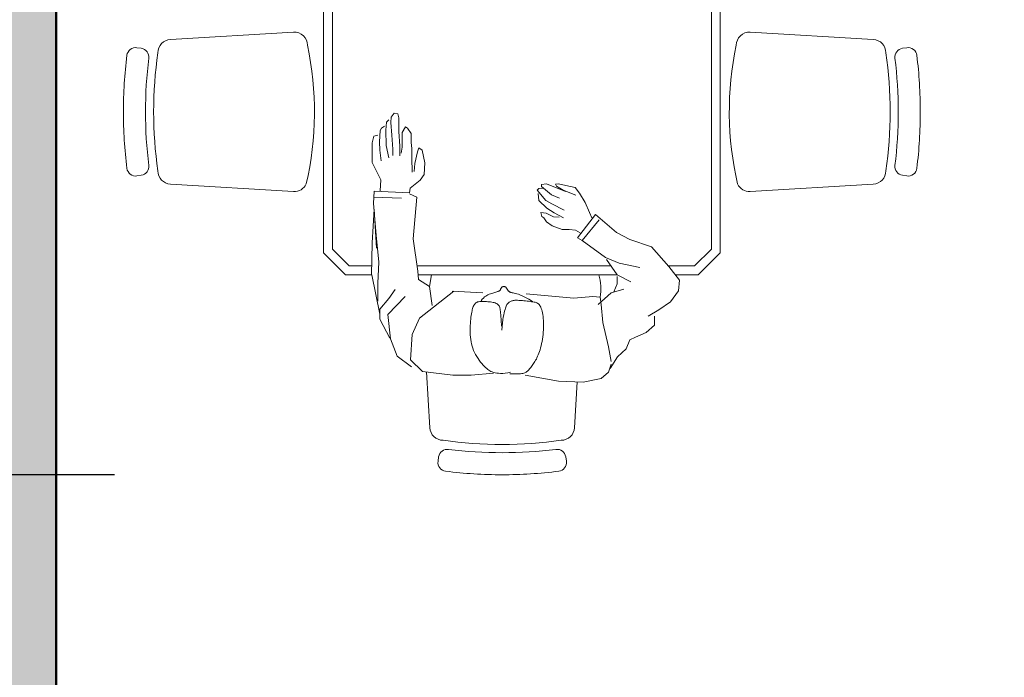
# Model space of a CAD drawing. Units: inches. Extents: x 1734 to 4011, y 1071 to 1891.
# Tile 19 of 27: x 3311 to 3379, y 1638 to 1683. Entities that reach past the tile are written whole.
import ezdxf

# ---------------------------------------------------------------- set-up
doc = ezdxf.new("R2010")
doc.units = ezdxf.units.IN
for name, color, linetype, lineweight in [('A-ANNO-DIMS', 2, 'Continuous', 18), ('A-FURN', 8, 'Continuous', 18), ('A-WALL', 7, 'Continuous', 50), ('A-WALL-PATT', 8, 'Continuous', 13)]:
    doc.layers.add(name, color=color, linetype=linetype, lineweight=lineweight)
doc.styles.get("Standard").update_dxf_attribs({"font": 'arial.ttf'})
doc.dimstyles.new('ISO-25', dxfattribs={"dimtxt": 5, "dimasz": 2.5, "dimexe": 1.25, "dimexo": 0.625, "dimtad": 1, "dimdec": 1, "dimlunit": 3, "dimtxsty": 'Standard', "dimcen": 2.5, "dimclrt": 1, "dimadec": 0, "dimazin": 0, "dimtfac": 1, "dimtdec": 1, "dimtmove": 0, "dimatfit": 3, "dimfxl": 1, "dimarcsym": 0})

# ---------------------------------------------------------------- blocks, each defined once
blk = doc.blocks.new('A$C421907B3')
for p, q in [((0.7079, 2.565), (0.7245, 2.5796)), ((0.7245, 2.5796), (0.7652, 2.5876)), ((0.7652, 2.5876), (0.8209, 2.5856)), ((0.8209, 2.5856), (0.8965, 2.5714)), ((0.9684, 2.5672), (1.0195, 2.5715)), ((1.0195, 2.5715), (1.0607, 2.5715)), ((1.0607, 2.5715), (1.1301, 2.5633)), ((0.7038, 2.5568), (0.6875, 2.5302)), ((0.7017, 2.5468), (0.7079, 2.565)), ((0.8792, 2.5478), (0.8777, 2.5455)), ((0.8808, 2.55), (0.8792, 2.5478)), ((0.8823, 2.5521), (0.8808, 2.55)), ((0.8839, 2.5541), (0.8823, 2.5521)), ((0.8853, 2.556), (0.8839, 2.5541)), ((0.8868, 2.5577), (0.8853, 2.556)), ((0.8883, 2.5594), (0.8868, 2.5577)), ((0.8897, 2.5609), (0.8883, 2.5594)), ((0.8911, 2.5623), (0.8897, 2.5609)), ((0.8926, 2.5635), (0.8911, 2.5623)), ((0.8941, 2.5647), (0.8926, 2.5635)), ((0.8958, 2.5657), (0.8941, 2.5647)), ((0.8976, 2.5665), (0.8958, 2.5657)), ((0.8996, 2.5672), (0.8976, 2.5665)), ((0.9018, 2.5678), (0.8996, 2.5672)), ((0.9043, 2.5682), (0.9018, 2.5678)), ((0.9071, 2.5684), (0.9043, 2.5682)), ((0.9102, 2.5686), (0.9071, 2.5684)), ((0.9137, 2.5687), (0.9102, 2.5686)), ((0.9175, 2.5687), (0.9137, 2.5687)), ((0.9217, 2.5687), (0.9175, 2.5687)), ((0.9264, 2.5687), (0.9217, 2.5687)), ((0.9314, 2.5687), (0.9264, 2.5687)), ((0.9361, 2.5662), (0.9297, 2.5647)), ((0.942, 2.5671), (0.9361, 2.5662)), ((0.9475, 2.5676), (0.942, 2.5671)), ((0.9525, 2.5677), (0.9475, 2.5676)), ((0.9571, 2.5675), (0.9525, 2.5677)), ((0.9614, 2.5669), (0.9571, 2.5675)), ((0.9652, 2.5662), (0.9614, 2.5669)), ((0.9686, 2.5653), (0.9652, 2.5662)), ((0.9717, 2.5643), (0.9686, 2.5653)), ((0.9745, 2.5632), (0.9717, 2.5643)), ((0.977, 2.5619), (0.9745, 2.5632)), ((0.9794, 2.5605), (0.977, 2.5619)), ((0.9818, 2.5588), (0.9794, 2.5605)), ((0.9841, 2.5568), (0.9818, 2.5588)), ((0.9865, 2.5545), (0.9841, 2.5568)), ((0.9891, 2.5519), (0.9865, 2.5545)), ((0.9918, 2.5489), (0.9891, 2.5519)), ((0.9948, 2.5455), (0.9918, 2.5489)), ((1.1301, 2.5633), (1.1567, 2.5368)), ((1.1546, 2.5531), (1.1875, 2.5285)), ((0.6875, 2.5302), (0.6672, 2.5117)), ((0.7017, 2.5405), (0.7079, 2.5077)), ((0.8669, 2.5256), (0.8655, 2.522)), ((0.8684, 2.5289), (0.8669, 2.5256)), ((0.8699, 2.5321), (0.8684, 2.5289)), ((0.8714, 2.5351), (0.8699, 2.5321)), ((0.873, 2.5379), (0.8714, 2.5351)), ((0.8745, 2.5405), (0.873, 2.5379)), ((0.8761, 2.543), (0.8745, 2.5405)), ((0.8777, 2.5455), (0.8761, 2.543)), ((0.9978, 2.5419), (0.9948, 2.5455)), ((1.0008, 2.5379), (0.9978, 2.5419)), ((1.0037, 2.5338), (1.0008, 2.5379)), ((1.0066, 2.5294), (1.0037, 2.5338)), ((1.0093, 2.5249), (1.0066, 2.5294)), ((1.1567, 2.5368), (1.153, 2.4792)), ((1.1875, 2.5285), (1.202, 2.4895)), ((0.6672, 2.5117), (0.6589, 2.4912)), ((0.7079, 2.5077), (0.7204, 2.4524)), ((0.8604, 2.5049), (0.8594, 2.5001)), ((0.8616, 2.5096), (0.8604, 2.5049)), ((0.8628, 2.514), (0.8616, 2.5096)), ((0.8641, 2.5181), (0.8628, 2.514)), ((0.8655, 2.522), (0.8641, 2.5181)), ((1.0117, 2.5203), (1.0093, 2.5249)), ((1.0138, 2.5155), (1.0117, 2.5203)), ((1.0156, 2.5107), (1.0138, 2.5155)), ((1.0171, 2.5058), (1.0156, 2.5107)), ((1.0184, 2.5008), (1.0171, 2.5058)), ((0.6464, 2.4852), (0.6219, 2.4749)), ((0.6589, 2.4912), (0.6464, 2.4852)), ((0.8568, 2.4847), (0.8562, 2.4794)), ((0.8576, 2.49), (0.8568, 2.4847)), ((0.8584, 2.4951), (0.8576, 2.49)), ((0.8594, 2.5001), (0.8584, 2.4951)), ((1.0194, 2.4958), (1.0184, 2.5008)), ((1.0202, 2.4907), (1.0194, 2.4958)), ((1.0208, 2.4855), (1.0202, 2.4907)), ((1.0212, 2.4802), (1.0208, 2.4855)), ((1.202, 2.4895), (1.2083, 2.4342)), ((1.2041, 2.4875), (1.2266, 2.4445)), ((0.6219, 2.4749), (0.6036, 2.4584)), ((0.6036, 2.4584), (0.6036, 2.4379)), ((0.8552, 2.4632), (0.8551, 2.4579)), ((0.8554, 2.4686), (0.8552, 2.4632)), ((0.8558, 2.474), (0.8554, 2.4686)), ((0.8562, 2.4794), (0.8558, 2.474)), ((0.9483, 2.453), (0.9491, 2.4609)), ((0.9491, 2.4609), (0.9498, 2.4698)), ((0.9505, 2.4603), (0.9511, 2.447)), ((1.021, 2.4541), (1.0212, 2.4591)), ((1.0214, 2.4749), (1.0212, 2.4802)), ((1.0212, 2.4591), (1.0214, 2.4643)), ((1.0215, 2.4696), (1.0214, 2.4749)), ((1.0214, 2.4643), (1.0215, 2.4696)), ((1.153, 2.4792), (1.1364, 2.4424)), ((0.6178, 2.4379), (0.5933, 2.4236)), ((0.7204, 2.4524), (0.7246, 2.4114)), ((0.8551, 2.4579), (0.8552, 2.4527)), ((0.8552, 2.4527), (0.8554, 2.4476)), ((0.8554, 2.4476), (0.8557, 2.4428)), ((0.8557, 2.4428), (0.8561, 2.4383)), ((0.8561, 2.4383), (0.8567, 2.4341)), ((0.9455, 2.4346), (0.9465, 2.4399)), ((0.9465, 2.4399), (0.9474, 2.446)), ((0.9474, 2.446), (0.9483, 2.453)), ((0.9511, 2.447), (0.9518, 2.4364)), ((0.9518, 2.4364), (0.9526, 2.4283)), ((1.0186, 2.4325), (1.0192, 2.4362)), ((1.0192, 2.4362), (1.0197, 2.4402)), ((1.0197, 2.4402), (1.0202, 2.4445)), ((1.0202, 2.4445), (1.0206, 2.4492)), ((1.0206, 2.4492), (1.021, 2.4541)), ((1.1364, 2.4424), (1.0587, 2.3808)), ((1.2266, 2.4445), (1.2266, 2.422)), ((0.5933, 2.4236), (0.5667, 2.4051)), ((0.8567, 2.4341), (0.8574, 2.4301)), ((0.8574, 2.4301), (0.8582, 2.4265)), ((0.8582, 2.4265), (0.8591, 2.4232)), ((0.8591, 2.4232), (0.8601, 2.4202)), ((0.8601, 2.4202), (0.8612, 2.4176)), ((0.8612, 2.4176), (0.8624, 2.4152)), ((0.8624, 2.4152), (0.8637, 2.4132)), ((0.9391, 2.4131), (0.9399, 2.415)), ((0.9399, 2.415), (0.9408, 2.4171)), ((0.9408, 2.4171), (0.9416, 2.4196)), ((0.9416, 2.4196), (0.9425, 2.4226)), ((0.9425, 2.4226), (0.9435, 2.426)), ((0.9435, 2.426), (0.9445, 2.43)), ((0.9445, 2.43), (0.9455, 2.4346)), ((0.9526, 2.4283), (0.9535, 2.4222)), ((0.9535, 2.4222), (0.9546, 2.4177)), ((0.9546, 2.4177), (0.9558, 2.4146)), ((0.9558, 2.4146), (0.9572, 2.4124)), ((1.0124, 2.4119), (1.0135, 2.4137)), ((1.0135, 2.4137), (1.0144, 2.4158)), ((1.0144, 2.4158), (1.0152, 2.418)), ((1.0152, 2.418), (1.016, 2.4204)), ((1.016, 2.4204), (1.0168, 2.423)), ((1.0168, 2.423), (1.0174, 2.4259)), ((1.0174, 2.4259), (1.0181, 2.429)), ((1.0181, 2.429), (1.0186, 2.4325)), ((1.1077, 2.4136), (1.114, 2.3706)), ((1.2083, 2.4342), (1.1693, 2.3932)), ((1.2266, 2.422), (1.2062, 2.3974)), ((1.2447, 2.3435), (1.2266, 2.4332)), ((0.5667, 2.4051), (0.5484, 2.3805)), ((0.7308, 2.4114), (0.7018, 2.3846)), ((0.7246, 2.4114), (0.7267, 2.3949)), ((0.7267, 2.3949), (0.7429, 2.3929)), ((0.7429, 2.3929), (0.7861, 2.3972)), ((0.7861, 2.3972), (0.8946, 2.387)), ((0.8637, 2.4132), (0.8651, 2.4114)), ((0.8651, 2.4114), (0.8666, 2.41)), ((0.8666, 2.41), (0.8682, 2.4088)), ((0.8682, 2.4088), (0.87, 2.4078)), ((0.87, 2.4078), (0.872, 2.407)), ((0.872, 2.407), (0.8742, 2.4063)), ((0.8742, 2.4063), (0.8767, 2.4058)), ((0.8767, 2.4058), (0.8794, 2.4052)), ((0.8794, 2.4052), (0.8824, 2.4048)), ((0.8801, 2.4042), (0.8884, 2.3992)), ((0.8824, 2.4048), (0.8857, 2.4043)), ((0.8857, 2.4043), (0.8891, 2.4039)), ((0.8884, 2.3992), (0.8957, 2.3952)), ((0.8891, 2.4039), (0.8925, 2.4035)), ((0.8925, 2.4035), (0.896, 2.4031)), ((0.8957, 2.3952), (0.9019, 2.3921)), ((0.896, 2.4031), (0.8995, 2.4027)), ((0.8995, 2.4027), (0.9028, 2.4024)), ((0.9019, 2.3921), (0.9073, 2.3897)), ((0.9028, 2.4024), (0.9059, 2.4022)), ((0.9059, 2.4022), (0.9088, 2.4019)), ((0.9088, 2.4019), (0.9114, 2.4018)), ((0.9114, 2.4018), (0.9138, 2.4016)), ((0.9138, 2.4016), (0.9161, 2.4016)), ((0.9161, 2.4016), (0.9182, 2.4016)), ((0.9182, 2.4016), (0.9201, 2.4017)), ((0.9201, 2.4017), (0.9219, 2.4019)), ((0.9219, 2.4019), (0.9237, 2.4022)), ((0.9237, 2.4022), (0.9254, 2.4026)), ((0.9254, 2.4026), (0.927, 2.4031)), ((0.927, 2.4031), (0.9286, 2.4037)), ((0.9286, 2.4037), (0.9301, 2.4044)), ((0.9301, 2.4044), (0.9315, 2.4052)), ((0.9315, 2.4052), (0.9329, 2.406)), ((0.9329, 2.406), (0.9341, 2.4069)), ((0.9341, 2.4069), (0.9353, 2.4079)), ((0.9353, 2.4079), (0.9363, 2.409)), ((0.9363, 2.409), (0.9373, 2.4102)), ((0.9373, 2.4102), (0.9382, 2.4116)), ((0.9382, 2.4116), (0.9391, 2.4131)), ((0.9572, 2.4124), (0.9588, 2.4109)), ((0.9588, 2.4109), (0.9606, 2.4096)), ((0.9606, 2.4096), (0.9626, 2.4086)), ((0.9626, 2.4086), (0.9647, 2.4077)), ((0.9647, 2.4077), (0.9671, 2.407)), ((0.9671, 2.407), (0.9696, 2.4064)), ((0.9696, 2.4064), (0.9722, 2.406)), ((0.9722, 2.406), (0.9751, 2.4055)), ((0.9751, 2.4055), (0.9781, 2.4052)), ((0.9781, 2.4052), (0.9812, 2.4048)), ((0.9812, 2.4048), (0.9844, 2.4045)), ((0.9837, 2.3905), (0.9863, 2.3922)), ((0.9844, 2.4045), (0.9877, 2.4043)), ((0.9863, 2.3922), (0.9889, 2.3941)), ((0.9877, 2.4043), (0.9909, 2.4041)), ((0.9889, 2.3941), (0.9915, 2.3965)), ((0.9909, 2.4041), (0.9941, 2.4041)), ((0.9915, 2.3965), (0.994, 2.3993)), ((0.994, 2.3993), (0.9965, 2.4026)), ((0.9941, 2.4041), (0.9971, 2.4042)), ((0.9971, 2.4042), (0.9999, 2.4044)), ((0.9999, 2.4044), (1.0025, 2.4049)), ((1.0025, 2.4049), (1.0047, 2.4055)), ((1.0047, 2.4055), (1.0067, 2.4064)), ((1.0067, 2.4064), (1.0085, 2.4075)), ((1.0085, 2.4075), (1.01, 2.4087)), ((1.01, 2.4087), (1.0113, 2.4102)), ((1.0113, 2.4102), (1.0124, 2.4119)), ((1.2062, 2.3974), (1.1917, 2.3769)), ((1.2308, 2.3624), (1.2308, 2.4035)), ((0.5484, 2.3805), (0.5463, 2.356)), ((0.7018, 2.3846), (0.6731, 2.3766)), ((0.6876, 2.3643), (0.6959, 2.3826)), ((0.9073, 2.3897), (0.9119, 2.3881)), ((0.9119, 2.3881), (0.9157, 2.3869)), ((0.9157, 2.3869), (0.919, 2.386)), ((0.919, 2.386), (0.9217, 2.3854)), ((0.9217, 2.3854), (0.924, 2.3849)), ((0.924, 2.3849), (0.926, 2.3844)), ((0.926, 2.3844), (0.9277, 2.384)), ((0.9277, 2.384), (0.929, 2.3837)), ((0.929, 2.3837), (0.9302, 2.3833)), ((0.9302, 2.3833), (0.9312, 2.383)), ((0.9312, 2.383), (0.932, 2.3826)), ((0.932, 2.3826), (0.9327, 2.3823)), ((0.9327, 2.3823), (0.9334, 2.3818)), ((0.9334, 2.3818), (0.934, 2.3813)), ((0.934, 2.3813), (0.9346, 2.3808)), ((0.9346, 2.3808), (0.9351, 2.3803)), ((0.9351, 2.3803), (0.9356, 2.3797)), ((0.9356, 2.3797), (0.936, 2.379)), ((0.936, 2.379), (0.9365, 2.3783)), ((0.9365, 2.3783), (0.9369, 2.3776)), ((0.9369, 2.3776), (0.9372, 2.3769)), ((0.9372, 2.3769), (0.9376, 2.3761)), ((0.9376, 2.3761), (0.938, 2.3753)), ((0.938, 2.3753), (0.9384, 2.3746)), ((0.9384, 2.3746), (0.9389, 2.3738)), ((0.9389, 2.3738), (0.9395, 2.3731)), ((0.9395, 2.3731), (0.9401, 2.3725)), ((0.9401, 2.3725), (0.9408, 2.3719)), ((0.9408, 2.3719), (0.9417, 2.3714)), ((0.9417, 2.3714), (0.9426, 2.371)), ((0.9426, 2.371), (0.9437, 2.3707)), ((0.9437, 2.3707), (0.9447, 2.3706)), ((0.9447, 2.3706), (0.9458, 2.3705)), ((0.9458, 2.3705), (0.9468, 2.3706)), ((0.9468, 2.3706), (0.9478, 2.3708)), ((0.9478, 2.3708), (0.9487, 2.3712)), ((0.9487, 2.3712), (0.9494, 2.3717)), ((0.9494, 2.3717), (0.9501, 2.3723)), ((0.9501, 2.3723), (0.9507, 2.3731)), ((0.9507, 2.3731), (0.9512, 2.3739)), ((0.9512, 2.3739), (0.9517, 2.3747)), ((0.9517, 2.3747), (0.9521, 2.3755)), ((0.9521, 2.3755), (0.9524, 2.3764)), ((0.9524, 2.3764), (0.9527, 2.3771)), ((0.9527, 2.3771), (0.953, 2.3778)), ((0.953, 2.3778), (0.9533, 2.3785)), ((0.9533, 2.3785), (0.9536, 2.379)), ((0.9536, 2.379), (0.954, 2.3796)), ((0.954, 2.3796), (0.9546, 2.3801)), ((0.9546, 2.3801), (0.9554, 2.3805)), ((0.9554, 2.3805), (0.9564, 2.381)), ((0.9564, 2.381), (0.9577, 2.3815)), ((0.9577, 2.3815), (0.9593, 2.382)), ((0.9593, 2.382), (0.9611, 2.3826)), ((0.9611, 2.3826), (0.9632, 2.3832)), ((0.9632, 2.3832), (0.9655, 2.3838)), ((0.9655, 2.3838), (0.9679, 2.3845)), ((0.9679, 2.3845), (0.9705, 2.3853)), ((0.9705, 2.3853), (0.9731, 2.3861)), ((0.9731, 2.3861), (0.9757, 2.387)), ((0.9757, 2.387), (0.9784, 2.388)), ((0.9784, 2.388), (0.9811, 2.3892)), ((0.9811, 2.3892), (0.9837, 2.3905)), ((0.9931, 2.3848), (1.0625, 2.3808)), ((1.114, 2.3706), (1.1095, 2.3436)), ((1.114, 2.3706), (1.1385, 2.3544)), ((0.5463, 2.356), (0.5709, 2.3252)), ((0.6569, 2.3601), (0.6876, 2.3438)), ((0.6876, 2.3478), (0.6876, 2.3643)), ((1.1385, 2.3544), (1.1406, 2.3358)), ((1.2287, 2.3154), (1.2308, 2.3624)), ((0.5709, 2.3252), (0.6099, 2.2802)), ((0.6835, 2.317), (0.6365, 2.3273)), ((0.6876, 2.3438), (0.7122, 2.3088)), ((1.1406, 2.3358), (1.151, 2.262)), ((0.7143, 2.3048), (0.6835, 2.317)), ((0.7674, 2.2656), (0.7143, 2.3048)), ((1.235, 2.2538), (1.2287, 2.3154)), ((0.6099, 2.2802), (0.659, 2.2637)), ((0.659, 2.2637), (0.6898, 2.2475)), ((0.7288, 2.2187), (0.7675, 2.2658)), ((0.7779, 2.2598), (0.7368, 2.2065)), ((0.7675, 2.2658), (0.7779, 2.2598)), ((1.151, 2.262), (1.1428, 2.1677)), ((0.6898, 2.2475), (0.7368, 2.2065)), ((0.7716, 2.2487), (0.7827, 2.2421)), ((0.7827, 2.2421), (0.7969, 2.2406)), ((0.7969, 2.2406), (0.8131, 2.2406)), ((0.8131, 2.2406), (0.8354, 2.2325)), ((1.2413, 2.1822), (1.235, 2.2538)), ((0.7509, 2.2021), (0.7458, 2.2146)), ((0.8094, 2.2146), (0.8309, 2.2028)), ((0.8324, 2.2124), (0.8198, 2.2132)), ((0.8494, 2.2036), (0.8324, 2.2124)), ((0.8354, 2.2325), (0.8487, 2.2236)), ((0.8487, 2.2236), (0.8546, 2.2147)), ((0.8546, 2.2147), (0.859, 2.211)), ((0.7606, 2.1798), (0.7509, 2.2021)), ((0.8079, 2.1969), (0.8361, 2.1828)), ((0.8309, 2.2028), (0.8472, 2.1925)), ((0.8472, 2.1925), (0.8658, 2.1747)), ((0.8613, 2.2021), (0.8494, 2.2036)), ((0.859, 2.211), (0.8613, 2.2021)), ((0.7732, 2.1583), (0.7606, 2.1798)), ((0.8191, 2.1695), (0.8369, 2.1621)), ((0.8361, 2.1828), (0.8502, 2.1747)), ((0.8502, 2.1747), (0.8695, 2.1518)), ((0.8658, 2.1747), (0.8672, 2.1591)), ((1.1428, 2.1677), (1.159, 2.1597)), ((1.1777, 2.1697), (1.2413, 2.1677)), ((1.2392, 2.1535), (1.2413, 2.1822)), ((0.7835, 2.1457), (0.7732, 2.1583)), ((0.7814, 2.1628), (0.8102, 2.1517)), ((0.8221, 2.1369), (0.7835, 2.1457)), ((0.848, 2.1369), (0.805, 2.1547)), ((0.8102, 2.1517), (0.8257, 2.1428)), ((0.8369, 2.1621), (0.8599, 2.1429)), ((0.8658, 2.1481), (0.8561, 2.1473)), ((0.8695, 2.1518), (0.8658, 2.1481)), ((1.158, 2.1467), (1.1354, 2.1286)), ((1.1595, 2.1573), (1.158, 2.1467)), ((1.1595, 2.1573), (1.2392, 2.1535)), ((1.226, 2.1528), (1.2245, 2.1279)), ((0.828, 2.1376), (0.8221, 2.1369)), ((0.8257, 2.1428), (0.828, 2.1376)), ((0.8599, 2.1384), (0.848, 2.1369)), ((0.8599, 2.1429), (0.8599, 2.1384)), ((1.1354, 2.1286), (1.1263, 2.1158)), ((1.2245, 2.1279), (1.2358, 2.1052)), ((1.1263, 2.1158), (1.1248, 2.0893)), ((1.1474, 2.0909), (1.149, 2.1089)), ((1.1535, 2.1105), (1.1536, 2.078)), ((1.2358, 2.1052), (1.2442, 2.0886)), ((1.1248, 2.0893), (1.1308, 2.0606)), ((1.1414, 2.0644), (1.1474, 2.0909)), ((1.2238, 2.0848), (1.2269, 2.0606)), ((1.2442, 2.0886), (1.2442, 2.0441)), ((1.1308, 2.0606), (1.1377, 2.0553)), ((1.1377, 2.0553), (1.1414, 2.0644)), ((1.1536, 2.078), (1.1543, 2.0568)), ((1.1543, 2.0568), (1.1551, 2.0432)), ((1.1762, 2.0539), (1.1784, 2.0674)), ((1.1815, 2.0735), (1.1815, 2.0516)), ((1.1974, 2.0584), (1.1974, 2.0727)), ((1.1996, 2.0267), (1.1974, 2.0584)), ((1.2064, 2.078), (1.2125, 2.0501)), ((1.2269, 2.0606), (1.2276, 2.0418)), ((1.1551, 2.0432), (1.1558, 2.0229)), ((1.1762, 2.0357), (1.1762, 2.0539)), ((1.1762, 2.0206), (1.1762, 2.0357)), ((1.1815, 2.0516), (1.1831, 2.0183)), ((1.2125, 2.0501), (1.2132, 2.0154)), ((1.2276, 2.0418), (1.2261, 2.0161)), ((1.2442, 2.0441), (1.2404, 2.029)), ((1.1558, 2.0229), (1.1641, 2.0108)), ((1.168, 2.0077), (1.1762, 2.0206)), ((1.1831, 2.0183), (1.1831, 1.9874)), ((1.2019, 1.9979), (1.1996, 2.0267)), ((1.2132, 2.0154), (1.2117, 1.9972)), ((1.2261, 2.0161), (1.223, 2.0108)), ((1.2404, 2.029), (1.2314, 2.0267)), ((1.1641, 2.0108), (1.168, 2.0077)), ((1.2012, 1.9859), (1.2019, 1.9979)), ((1.2117, 1.9972), (1.2064, 1.9919)), ((1.223, 2.0108), (1.2163, 2.0063)), ((1.1831, 1.9874), (1.186, 1.9783)), ((1.186, 1.9783), (1.1944, 1.9768)), ((1.1944, 1.9768), (1.2012, 1.9859))]:
    blk.add_line(p, q)
at = {"ltscale": 0.1}
for points in [[(0.9489, 2.7478, 0.030867), (0.827, 2.7403, -0.408428), (0.8047, 2.7573), (0.8033, 2.7672, -0.419966), (0.8206, 2.7899, -0.030916), (0.9489, 2.7978, -0.030916), (1.0772, 2.7899, -0.419966), (1.0945, 2.7672), (1.0931, 2.7573, -0.408428), (1.0708, 2.7403, 0.030867)], [(0.0782, 2.1079, -0.399285), (0.1067, 2.1378), (0.3861, 2.1548, -0.305593), (0.4148, 2.1375, -0.109362), (0.4176, 1.8225, -0.429301), (0.3861, 1.7925), (0.1067, 1.8094, -0.399285), (0.0782, 1.8394, -0.071734)], [(1.7302, 2.1079, 0.399285), (1.7017, 2.1378), (1.4223, 2.1548, 0.305593), (1.3936, 2.1375, 0.109362), (1.3908, 1.8225, 0.429301), (1.4223, 1.7925), (1.7017, 1.8094, 0.399285), (1.7302, 1.8394, 0.071734)], [(0.05, 1.9736, 0.030867), (0.0575, 1.8517, -0.408428), (0.0405, 1.8294), (0.0306, 1.828, -0.419966), (0.0079, 1.8453, -0.030916), (0, 1.9736, -0.030916), (0.0079, 2.1019, -0.419966), (0.0306, 2.1193), (0.0405, 2.1178, -0.408428), (0.0575, 2.0956, 0.030867)], [(1.7584, 1.9736, -0.030867), (1.7509, 1.8517, 0.408428), (1.7679, 1.8294), (1.7778, 1.828, 0.419966), (1.8005, 1.8453, 0.030916), (1.8084, 1.9736, 0.030916), (1.8005, 2.1019, 0.419966), (1.7778, 2.1193), (1.7679, 2.1178, 0.408428), (1.7509, 2.0956, -0.030867)]]:
    blk.add_lwpolyline(points, format="xyb", close=True, dxfattribs=at)
blk.add_lwpolyline([(0.7784, 2.5871), (0.7847, 2.6911, -0.399285), (0.8147, 2.7196, -0.071734), (1.0831, 2.7196, -0.399285), (1.1131, 2.6911), (1.1208, 2.5644)], format="xyb", dxfattribs=at)
for points in [[(0.4542, 1.2262), (0.4542, 2.2936), (0.5042, 2.3436), (0.5562, 2.3436)], [(0.6878, 2.3436), (1.1397, 2.3436)], [(1.2446, 2.3436), (1.3042, 2.3436), (1.3542, 2.2936), (1.3542, 1.0533)], [(0.4742, 1.2101), (0.4742, 2.2853), (0.5125, 2.3236), (0.5723, 2.3236)], [(0.7018, 2.3236), (1.1423, 2.3236)], [(1.245, 2.3234), (1.2959, 2.3236), (1.3342, 2.2853), (1.3342, 1.0419)]]:
    blk.add_lwpolyline(points, dxfattribs=at)
blk.add_lwpolyline([(1.2332, 2.2712), (1.2341, 2.2831), (1.2396, 2.1946), (1.2396, 2.1946), (1.2419, 2.2332), (1.2437, 2.2711), (1.2448, 2.3081), (1.2452, 2.3436)])
blk.add_arc((0.8297, 2.3756), 0.1048, 169.4107, 197.7809)
blk = doc.blocks.new('*D99')
at = {"layer": 'A-ANNO-DIMS', "color": 0, "lineweight": -2, "transparency": 16777216}
for p, q in [((3317.994, 1736.234), (3304.669, 1736.234)), ((3305.919, 1733.734), (3305.919, 1654.07)), ((3317.994, 1651.57), (3304.669, 1651.57)), ((3305.919, 1651.57), (3305.919, 1564.027))]:
    blk.add_line(p, q, dxfattribs=at)
at = {"layer": 'A-ANNO-DIMS', "color": 0, "transparency": 16777216}
for points in [[(3305.503, 1733.734), (3306.336, 1733.734), (3305.919, 1736.234)], [(3305.503, 1654.07), (3306.336, 1654.07), (3305.919, 1651.57)]]:
    blk.add_solid(points, dxfattribs=at)
at = {"layer": 'Defpoints', "color": 0, "transparency": 16777216}
for p in [(3318.619, 1736.234), (3305.919, 1651.57), (3318.619, 1651.57)]:
    blk.add_point(p, dxfattribs=at)
at = {"layer": 'A-ANNO-DIMS', "color": 1, "transparency": 16777216, "insert": (3302.709, 1606.548), "char_height": 5, "attachment_point": 5, "rotation": 90}
blk.add_mtext('DINING SET 7\'-0 1/2" TYP.', dxfattribs=at)

msp = doc.modelspace()

# ---------------------------------------------------------------- hatches: boundary and pattern name
at = {"layer": 'A-WALL-PATT'}
h = msp.add_hatch(color=256, dxfattribs=at)
h.dxf.hatch_style = 1
h.paths.add_polyline_path([(3475.994, 1831.819), (3115.994, 1831.819), (3115.994, 1745.819), (3130.994, 1745.819), (3130.994, 1750.819), (3124.994, 1750.819), (3124.994, 1822.819), (3214.994, 1822.819), (3214.994, 1780.819), (3219.994, 1780.819), (3219.994, 1822.819), (3308.994, 1822.819), (3308.994, 1750.819), (3254.994, 1750.819), (3254.994, 1745.819), (3308.994, 1745.819), (3308.994, 1604.819), (3313.994, 1604.819), (3313.994, 1745.819), (3366.994, 1745.819), (3366.994, 1750.819), (3313.994, 1750.819), (3313.994, 1822.819), (3401.994, 1822.819), (3401.994, 1750.819), (3396.994, 1750.819), (3396.994, 1745.819), (3411.994, 1745.819), (3411.994, 1750.819), (3406.994, 1750.819), (3406.994, 1822.819), (3466.994, 1822.819), (3466.994, 1750.819), (3441.994, 1750.819), (3441.994, 1745.819), (3466.994, 1745.819), (3466.994, 1517.819), (3452.494, 1517.819), (3452.494, 1512.819), (3466.994, 1512.819), (3466.994, 1458.819), (3446.494, 1458.819), (3446.494, 1453.819), (3466.994, 1453.819), (3466.994, 1237.819), (3372.994, 1237.819), (3372.994, 1228.819), (3466.994, 1228.819), (3466.994, 1120.819), (3309.994, 1120.819), (3309.994, 1184.819), (3310.994, 1184.819), (3310.994, 1189.819), (3303.994, 1189.819), (3303.994, 1120.819), (3291.994, 1120.819), (3291.994, 1111.819), (3475.994, 1111.819)])
h.paths.add_polyline_path([(3169.994, 1745.819), (3224.994, 1745.819), (3224.994, 1750.819), (3154.994, 1750.819), (3154.994, 1745.819), (3160.994, 1745.819), (3160.994, 1636.819), (3169.994, 1636.819)], flags=17)
h.paths.add_polyline_path([(3169.994, 1588.819), (3160.994, 1588.819), (3160.994, 1559.819), (3313.994, 1559.819), (3313.994, 1568.819), (3308.994, 1568.819), (3308.994, 1564.819), (3169.994, 1564.819)], flags=17)
h.paths.add_polyline_path([(3416.494, 1517.819), (3401.994, 1517.819), (3401.994, 1512.819), (3416.494, 1512.819)], flags=17)
h.paths.add_polyline_path([(3371.994, 1517.819), (3366.994, 1517.819), (3366.994, 1453.819), (3392.494, 1453.819), (3392.494, 1458.819), (3371.994, 1458.819)], flags=17)
h.paths.add_polyline_path([(3258.994, 1529.819), (3160.994, 1529.819), (3160.994, 1494.819), (3169.994, 1494.819), (3169.994, 1524.819), (3253.994, 1524.819), (3253.994, 1520.819), (3258.994, 1520.819)], flags=17)
h.paths.add_polyline_path([(3263.994, 1458.819), (3258.994, 1458.819), (3258.994, 1490.819), (3253.994, 1490.819), (3253.994, 1458.819), (3169.994, 1458.819), (3169.994, 1470.819), (3160.994, 1470.819), (3160.994, 1387.819), (3169.994, 1387.819), (3169.994, 1453.819), (3263.994, 1453.819)], flags=17)
h.paths.add_polyline_path([(3313.994, 1453.819), (3318.994, 1453.819), (3318.994, 1458.819), (3299.994, 1458.819), (3299.994, 1453.819), (3308.994, 1453.819), (3308.994, 1321.819), (3266.494, 1321.819), (3266.494, 1312.819), (3313.994, 1312.819)], flags=17)
h.paths.add_polyline_path([(3212.494, 1321.819), (3169.994, 1321.819), (3169.994, 1339.819), (3160.994, 1339.819), (3160.994, 1312.819), (3212.494, 1312.819)], flags=17)
h.paths.add_polyline_path([(3313.994, 1288.819), (3304.994, 1288.819), (3304.994, 1285.819), (3313.994, 1285.819)], flags=17)
h.paths.add_polyline_path([(3324.994, 1237.819), (3304.994, 1237.819), (3304.994, 1228.819), (3324.994, 1228.819)], flags=17)

# ---------------------------------------------------------------- linework, layer by layer
at = {"layer": 'A-WALL'}
msp.add_line((3313.994, 1604.819), (3313.994, 1745.819), dxfattribs=at)

# ---------------------------------------------------------------- block references
at = {"layer": 'A-FURN', "xscale": 30.26057373645948, "yscale": 30.26057373645948, "zscale": 30.26057373645948, "rotation": 180}
msp.add_blockref('A$C421907B3', (3373.342, 1736.234), dxfattribs=at)

# ---------------------------------------------------------------- dimensions: what is measured, and where the dimension line sits
at = {"layer": 'A-ANNO-DIMS'}
dim = msp.add_linear_dim(base=(3305.919, 1651.57), p1=(3318.619, 1736.234), p2=(3318.619, 1651.57), angle=270, text='DINING SET <> TYP.', dimstyle='ISO-25', override={"dimdec": 1, "dimrnd": 0, "dimzin": 1, "dimlunit": 4, "dimfrac": 2}, dxfattribs=at)
dim.commit()
dim.dimension.update_dxf_attribs({"geometry": '*D99', "text_midpoint": (3302.709, 1606.548)})

doc.saveas('drawing.dxf')
